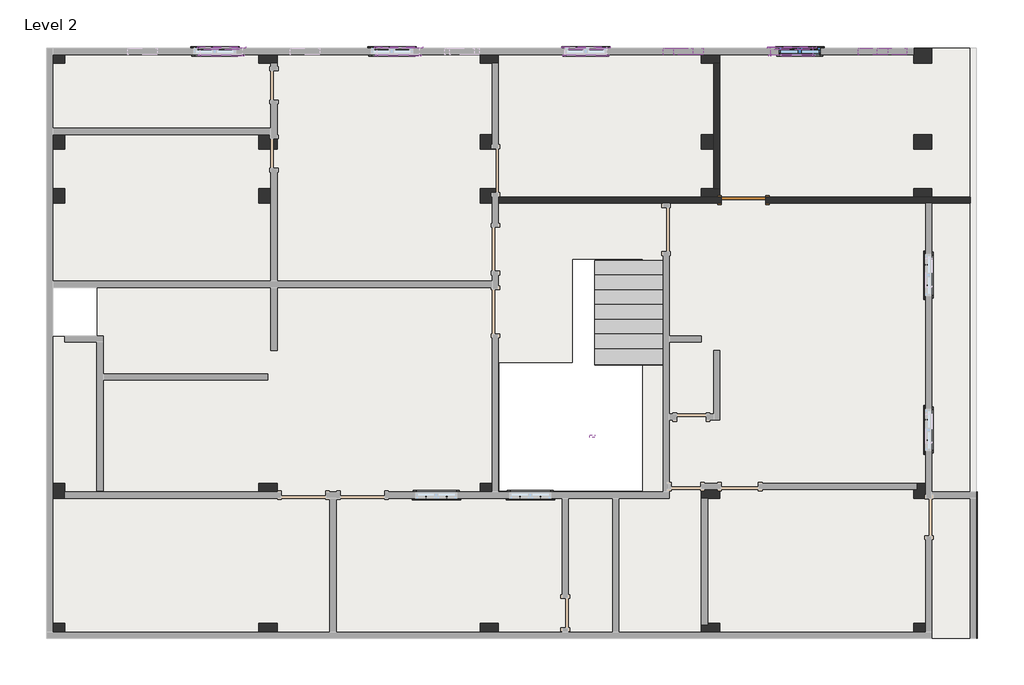
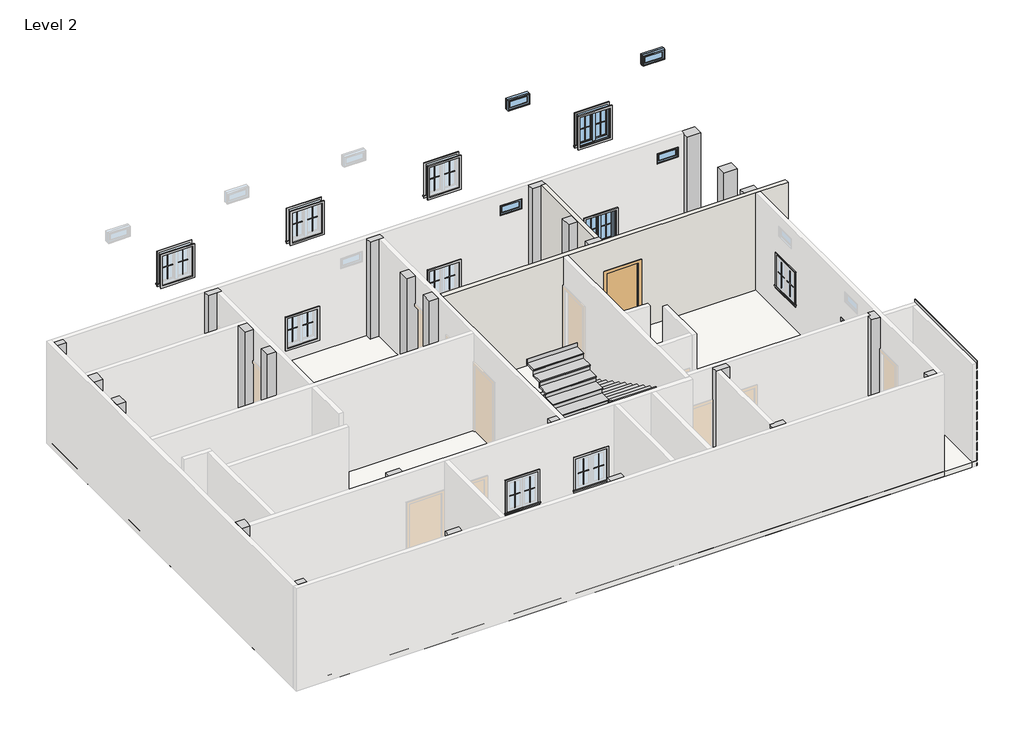
# One storey, part 2 of 2: 48 proxies, 25 columns, 6 windows, 2 walls, 1 air terminal, 1 door, 1 member, 1 slab, 1 stair flight.
"""IFC4 building model written with IfcOpenShell, lengths in millimetres."""

from ifc_helpers import new_model, si_unit, frame, origin, place, context, project, spatial, polyline, outline, extrude, faceted_brep, transform, mapped, element, save
from components import air_terminals_1_air_terminals_1_05a11ed2, muntin_pattern_2x2_muntin_pattern_2x2_b3fe6957, muntin_pattern_2x2_muntin_pattern_2x2_3e0ecaf2, trim_window_exterior_flat_with_sill_41619996, trim_window_interior_flat_picture_frame_51c85655, door_a3eb833a, stair_flight_69588459, window_4c2727af, window_0d9958e7

model = new_model("IFC4")

# Units and contexts
model_context = context("Model", 3, world=origin())
ifc_project = project(units=[si_unit("LENGTHUNIT", "METRE", prefix="MILLI")], contexts=[model_context])

# Site, building, storey
site = spatial("IfcSite", under=ifc_project)
building = spatial("IfcBuilding", under=site)
storey = spatial("IfcBuildingStorey", under=building, Name="Level 2", Elevation=3048.0)

# Air terminal
placement = place(None, origin())
air_terminals_1_air_terminals_1_shape = air_terminals_1_air_terminals_1_05a11ed2(model_context)
element("IfcAirTerminal", 1, ObjectType="Air Terminals 1 : Air Terminals 1", at=placement, inside=storey, context=model_context, shape_type="MappedRepresentation", body=[
    mapped(air_terminals_1_air_terminals_1_shape, transform((0.0, 0.0, 0.0), x_axis=(1.0, 0.0, 0.0), y_axis=(0.0, 1.0, 0.0), z_axis=(0.0, 0.0, 1.0))),
])

# Proxies
muntin_pattern_2x2_muntin_pattern_2x2_shape = muntin_pattern_2x2_muntin_pattern_2x2_b3fe6957(model_context)
element("IfcBuildingElementProxy", 2, Name="Muntin Pattern_2x2 : Muntin Pattern_2x2", ObjectType="Muntin Pattern_2x2 : Muntin Pattern_2x2", at=placement, inside=storey, context=model_context, shape_type="MappedRepresentation", body=[
    mapped(muntin_pattern_2x2_muntin_pattern_2x2_shape, transform((-4178.9300534, -6055.6581508, 4032.25), x_axis=(-1.0, 0.0, 0.0), y_axis=(0.0, -1.0, 0.0), z_axis=(0.0, 0.0, 1.0))),
])
element("IfcBuildingElementProxy", 3, Name="Muntin Pattern_2x2 : Muntin Pattern_2x2", ObjectType="Muntin Pattern_2x2 : Muntin Pattern_2x2", at=placement, inside=storey, context=model_context, shape_type="MappedRepresentation", body=[
    mapped(muntin_pattern_2x2_muntin_pattern_2x2_shape, transform((-2238.8239737, -6055.6581508, 4032.25), x_axis=(-1.0, 0.0, 0.0), y_axis=(0.0, -1.0, 0.0), z_axis=(0.0, 0.0, 1.0))),
])
element("IfcBuildingElementProxy", 4, Name="Muntin Pattern_2x2 : Muntin Pattern_2x2", ObjectType="Muntin Pattern_2x2 : Muntin Pattern_2x2", at=placement, inside=storey, context=model_context, shape_type="MappedRepresentation", body=[
    mapped(muntin_pattern_2x2_muntin_pattern_2x2_shape, transform((5725.4824466, -4869.7956508, 4032.25), x_axis=(0.0, 1.0, 0.0), y_axis=(-1.0, 0.0, 0.0), z_axis=(0.0, 0.0, 1.0))),
])
element("IfcBuildingElementProxy", 5, Name="Muntin Pattern_2x2 : Muntin Pattern_2x2", ObjectType="Muntin Pattern_2x2 : Muntin Pattern_2x2", at=placement, inside=storey, context=model_context, shape_type="MappedRepresentation", body=[
    mapped(muntin_pattern_2x2_muntin_pattern_2x2_shape, transform((5725.4824466, -1669.3956508, 4032.25), x_axis=(0.0, 1.0, 0.0), y_axis=(-1.0, 0.0, 0.0), z_axis=(0.0, 0.0, 1.0))),
])
element("IfcBuildingElementProxy", 6, Name="Muntin Pattern_2x2 : Muntin Pattern_2x2", ObjectType="Muntin Pattern_2x2 : Muntin Pattern_2x2", at=placement, inside=storey, context=model_context, shape_type="MappedRepresentation", body=[
    mapped(muntin_pattern_2x2_muntin_pattern_2x2_shape, transform((2733.0449466, 3221.6918492, 6774.3523039), x_axis=(1.0, 0.0, 0.0), y_axis=(0.0, 1.0, 0.0), z_axis=(0.0, 0.0, 1.0))),
])
element("IfcBuildingElementProxy", 7, Name="Muntin Pattern_2x2 : Muntin Pattern_2x2", ObjectType="Muntin Pattern_2x2 : Muntin Pattern_2x2", at=placement, inside=storey, context=model_context, shape_type="MappedRepresentation", body=[
    mapped(muntin_pattern_2x2_muntin_pattern_2x2_shape, transform((-1521.092894, 3221.6918492, 6774.3523039), x_axis=(1.0, 0.0, 0.0), y_axis=(0.0, 1.0, 0.0), z_axis=(0.0, 0.0, 1.0))),
])
element("IfcBuildingElementProxy", 8, Name="Muntin Pattern_2x2 : Muntin Pattern_2x2", ObjectType="Muntin Pattern_2x2 : Muntin Pattern_2x2", at=placement, inside=storey, context=model_context, shape_type="MappedRepresentation", body=[
    mapped(muntin_pattern_2x2_muntin_pattern_2x2_shape, transform((-1521.092894, 3221.6918492, 3670.3), x_axis=(1.0, 0.0, 0.0), y_axis=(0.0, 1.0, 0.0), z_axis=(0.0, 0.0, 1.0))),
])
element("IfcBuildingElementProxy", 9, Name="Muntin Pattern_2x2 : Muntin Pattern_2x2", ObjectType="Muntin Pattern_2x2 : Muntin Pattern_2x2", at=placement, inside=storey, context=model_context, shape_type="MappedRepresentation", body=[
    mapped(muntin_pattern_2x2_muntin_pattern_2x2_shape, transform((2898.507106, 3221.6918492, 3670.3), x_axis=(1.0, 0.0, 0.0), y_axis=(0.0, 1.0, 0.0), z_axis=(0.0, 0.0, 1.0))),
])
element("IfcBuildingElementProxy", 10, Name="Muntin Pattern_2x2 : Muntin Pattern_2x2", ObjectType="Muntin Pattern_2x2 : Muntin Pattern_2x2", at=placement, inside=storey, context=model_context, shape_type="MappedRepresentation", body=[
    mapped(muntin_pattern_2x2_muntin_pattern_2x2_shape, transform((-5391.7800534, 3221.6918492, 6774.3523039), x_axis=(1.0, 0.0, 0.0), y_axis=(0.0, 1.0, 0.0), z_axis=(0.0, 0.0, 1.0))),
])
element("IfcBuildingElementProxy", 11, Name="Muntin Pattern_2x2 : Muntin Pattern_2x2", ObjectType="Muntin Pattern_2x2 : Muntin Pattern_2x2", at=placement, inside=storey, context=model_context, shape_type="MappedRepresentation", body=[
    mapped(muntin_pattern_2x2_muntin_pattern_2x2_shape, transform((-9049.3800534, 3221.6918492, 6774.3523039), x_axis=(1.0, 0.0, 0.0), y_axis=(0.0, 1.0, 0.0), z_axis=(0.0, 0.0, 1.0))),
])
element("IfcBuildingElementProxy", 12, Name="Muntin Pattern_2x2 : Muntin Pattern_2x2", ObjectType="Muntin Pattern_2x2 : Muntin Pattern_2x2", at=placement, inside=storey, context=model_context, shape_type="MappedRepresentation", body=[
    mapped(muntin_pattern_2x2_muntin_pattern_2x2_shape, transform((-5525.1300534, 3221.6918492, 3670.3), x_axis=(1.0, 0.0, 0.0), y_axis=(0.0, 1.0, 0.0), z_axis=(0.0, 0.0, 1.0))),
])
element("IfcBuildingElementProxy", 13, Name="Muntin Pattern_2x2 : Muntin Pattern_2x2", ObjectType="Muntin Pattern_2x2 : Muntin Pattern_2x2", at=placement, inside=storey, context=model_context, shape_type="MappedRepresentation", body=[
    mapped(muntin_pattern_2x2_muntin_pattern_2x2_shape, transform((-9182.7300534, 3221.6918492, 3670.3), x_axis=(1.0, 0.0, 0.0), y_axis=(0.0, 1.0, 0.0), z_axis=(0.0, 0.0, 1.0))),
])
muntin_pattern_2x2_muntin_pattern_2x2_2_shape = muntin_pattern_2x2_muntin_pattern_2x2_3e0ecaf2(model_context)
element("IfcBuildingElementProxy", 14, Name="Muntin Pattern_2x2 : Muntin Pattern_2x2", ObjectType="Muntin Pattern_2x2 : Muntin Pattern_2x2", at=placement, inside=storey, context=model_context, shape_type="MappedRepresentation", body=[
    mapped(muntin_pattern_2x2_muntin_pattern_2x2_2_shape, transform((-4607.5550534, -6055.6581508, 4032.25), x_axis=(1.0, 0.0, 0.0), y_axis=(0.0, 1.0, 0.0), z_axis=(0.0, 0.0, 1.0))),
])
element("IfcBuildingElementProxy", 15, Name="Muntin Pattern_2x2 : Muntin Pattern_2x2", ObjectType="Muntin Pattern_2x2 : Muntin Pattern_2x2", at=placement, inside=storey, context=model_context, shape_type="MappedRepresentation", body=[
    mapped(muntin_pattern_2x2_muntin_pattern_2x2_2_shape, transform((-2667.4489737, -6055.6581508, 4032.25), x_axis=(1.0, 0.0, 0.0), y_axis=(0.0, 1.0, 0.0), z_axis=(0.0, 0.0, 1.0))),
])
element("IfcBuildingElementProxy", 16, Name="Muntin Pattern_2x2 : Muntin Pattern_2x2", ObjectType="Muntin Pattern_2x2 : Muntin Pattern_2x2", at=placement, inside=storey, context=model_context, shape_type="MappedRepresentation", body=[
    mapped(muntin_pattern_2x2_muntin_pattern_2x2_2_shape, transform((5725.4824466, -4441.1706508, 4032.25), x_axis=(0.0, -1.0, 0.0), y_axis=(1.0, 0.0, 0.0), z_axis=(0.0, 0.0, 1.0))),
])
element("IfcBuildingElementProxy", 17, Name="Muntin Pattern_2x2 : Muntin Pattern_2x2", ObjectType="Muntin Pattern_2x2 : Muntin Pattern_2x2", at=placement, inside=storey, context=model_context, shape_type="MappedRepresentation", body=[
    mapped(muntin_pattern_2x2_muntin_pattern_2x2_2_shape, transform((5725.4824466, -1240.7706508, 4032.25), x_axis=(0.0, -1.0, 0.0), y_axis=(1.0, 0.0, 0.0), z_axis=(0.0, 0.0, 1.0))),
])
element("IfcBuildingElementProxy", 18, Name="Muntin Pattern_2x2 : Muntin Pattern_2x2", ObjectType="Muntin Pattern_2x2 : Muntin Pattern_2x2", at=placement, inside=storey, context=model_context, shape_type="MappedRepresentation", body=[
    mapped(muntin_pattern_2x2_muntin_pattern_2x2_2_shape, transform((3161.6699466, 3221.6918492, 6774.3523039), x_axis=(-1.0, 0.0, 0.0), y_axis=(0.0, -1.0, 0.0), z_axis=(0.0, 0.0, 1.0))),
])
element("IfcBuildingElementProxy", 19, Name="Muntin Pattern_2x2 : Muntin Pattern_2x2", ObjectType="Muntin Pattern_2x2 : Muntin Pattern_2x2", at=placement, inside=storey, context=model_context, shape_type="MappedRepresentation", body=[
    mapped(muntin_pattern_2x2_muntin_pattern_2x2_2_shape, transform((-1092.467894, 3221.6918492, 6774.3523039), x_axis=(-1.0, 0.0, 0.0), y_axis=(0.0, -1.0, 0.0), z_axis=(0.0, 0.0, 1.0))),
])
element("IfcBuildingElementProxy", 20, Name="Muntin Pattern_2x2 : Muntin Pattern_2x2", ObjectType="Muntin Pattern_2x2 : Muntin Pattern_2x2", at=placement, inside=storey, context=model_context, shape_type="MappedRepresentation", body=[
    mapped(muntin_pattern_2x2_muntin_pattern_2x2_2_shape, transform((-1092.467894, 3221.6918492, 3670.3), x_axis=(-1.0, 0.0, 0.0), y_axis=(0.0, -1.0, 0.0), z_axis=(0.0, 0.0, 1.0))),
])
element("IfcBuildingElementProxy", 21, Name="Muntin Pattern_2x2 : Muntin Pattern_2x2", ObjectType="Muntin Pattern_2x2 : Muntin Pattern_2x2", at=placement, inside=storey, context=model_context, shape_type="MappedRepresentation", body=[
    mapped(muntin_pattern_2x2_muntin_pattern_2x2_2_shape, transform((3327.132106, 3221.6918492, 3670.3), x_axis=(-1.0, 0.0, 0.0), y_axis=(0.0, -1.0, 0.0), z_axis=(0.0, 0.0, 1.0))),
])
element("IfcBuildingElementProxy", 22, Name="Muntin Pattern_2x2 : Muntin Pattern_2x2", ObjectType="Muntin Pattern_2x2 : Muntin Pattern_2x2", at=placement, inside=storey, context=model_context, shape_type="MappedRepresentation", body=[
    mapped(muntin_pattern_2x2_muntin_pattern_2x2_2_shape, transform((-4963.1550534, 3221.6918492, 6774.3523039), x_axis=(-1.0, 0.0, 0.0), y_axis=(0.0, -1.0, 0.0), z_axis=(0.0, 0.0, 1.0))),
])
element("IfcBuildingElementProxy", 23, Name="Muntin Pattern_2x2 : Muntin Pattern_2x2", ObjectType="Muntin Pattern_2x2 : Muntin Pattern_2x2", at=placement, inside=storey, context=model_context, shape_type="MappedRepresentation", body=[
    mapped(muntin_pattern_2x2_muntin_pattern_2x2_2_shape, transform((-8620.7550534, 3221.6918492, 6774.3523039), x_axis=(-1.0, 0.0, 0.0), y_axis=(0.0, -1.0, 0.0), z_axis=(0.0, 0.0, 1.0))),
])
element("IfcBuildingElementProxy", 24, Name="Muntin Pattern_2x2 : Muntin Pattern_2x2", ObjectType="Muntin Pattern_2x2 : Muntin Pattern_2x2", at=placement, inside=storey, context=model_context, shape_type="MappedRepresentation", body=[
    mapped(muntin_pattern_2x2_muntin_pattern_2x2_2_shape, transform((-5096.5050534, 3221.6918492, 3670.3), x_axis=(-1.0, 0.0, 0.0), y_axis=(0.0, -1.0, 0.0), z_axis=(0.0, 0.0, 1.0))),
])
element("IfcBuildingElementProxy", 25, Name="Muntin Pattern_2x2 : Muntin Pattern_2x2", ObjectType="Muntin Pattern_2x2 : Muntin Pattern_2x2", at=placement, inside=storey, context=model_context, shape_type="MappedRepresentation", body=[
    mapped(muntin_pattern_2x2_muntin_pattern_2x2_2_shape, transform((-8754.1050534, 3221.6918492, 3670.3), x_axis=(-1.0, 0.0, 0.0), y_axis=(0.0, -1.0, 0.0), z_axis=(0.0, 0.0, 1.0))),
])
trim_window_exterior_flat_with_sill_shape = trim_window_exterior_flat_with_sill_41619996(model_context)
element("IfcBuildingElementProxy", 26, Name="Trim-Window-Exterior-Flat : with Sill", ObjectType="Trim-Window-Exterior-Flat : with Sill", at=placement, inside=storey, context=model_context, shape_type="MappedRepresentation", body=[
    mapped(trim_window_exterior_flat_with_sill_shape, transform((-4393.2425534, -6065.1831508, 4876.8), x_axis=(1.0, 0.0, 0.0), y_axis=(0.0, 0.0, 1.0), z_axis=(0.0, -1.0, 0.0))),
])
element("IfcBuildingElementProxy", 27, Name="Trim-Window-Exterior-Flat : with Sill", ObjectType="Trim-Window-Exterior-Flat : with Sill", at=placement, inside=storey, context=model_context, shape_type="MappedRepresentation", body=[
    mapped(trim_window_exterior_flat_with_sill_shape, transform((-2453.1364737, -6065.1831508, 4876.8), x_axis=(1.0, 0.0, 0.0), y_axis=(0.0, 0.0, 1.0), z_axis=(0.0, -1.0, 0.0))),
])
element("IfcBuildingElementProxy", 28, Name="Trim-Window-Exterior-Flat : with Sill", ObjectType="Trim-Window-Exterior-Flat : with Sill", at=placement, inside=storey, context=model_context, shape_type="MappedRepresentation", body=[
    mapped(trim_window_exterior_flat_with_sill_shape, transform((5715.9574466, -4655.4831508, 4876.8), x_axis=(0.0, -1.0, 0.0), y_axis=(0.0, 0.0, 1.0), z_axis=(-1.0, 0.0, 0.0))),
])
element("IfcBuildingElementProxy", 29, Name="Trim-Window-Exterior-Flat : with Sill", ObjectType="Trim-Window-Exterior-Flat : with Sill", at=placement, inside=storey, context=model_context, shape_type="MappedRepresentation", body=[
    mapped(trim_window_exterior_flat_with_sill_shape, transform((5715.9574466, -1455.0831508, 4876.8), x_axis=(0.0, -1.0, 0.0), y_axis=(0.0, 0.0, 1.0), z_axis=(-1.0, 0.0, 0.0))),
])
element("IfcBuildingElementProxy", 30, Name="Trim-Window-Exterior-Flat : with Sill", ObjectType="Trim-Window-Exterior-Flat : with Sill", at=placement, inside=storey, context=model_context, shape_type="MappedRepresentation", body=[
    mapped(trim_window_exterior_flat_with_sill_shape, transform((2947.3574466, 3231.2168492, 7618.9023039), x_axis=(-1.0, 0.0, 0.0), y_axis=(0.0, 0.0, 1.0), z_axis=(0.0, 1.0, 0.0))),
])
element("IfcBuildingElementProxy", 31, Name="Trim-Window-Exterior-Flat : with Sill", ObjectType="Trim-Window-Exterior-Flat : with Sill", at=placement, inside=storey, context=model_context, shape_type="MappedRepresentation", body=[
    mapped(trim_window_exterior_flat_with_sill_shape, transform((-1306.780394, 3231.2168492, 7618.9023039), x_axis=(-1.0, 0.0, 0.0), y_axis=(0.0, 0.0, 1.0), z_axis=(0.0, 1.0, 0.0))),
])
element("IfcBuildingElementProxy", 32, Name="Trim-Window-Exterior-Flat : with Sill", ObjectType="Trim-Window-Exterior-Flat : with Sill", at=placement, inside=storey, context=model_context, shape_type="MappedRepresentation", body=[
    mapped(trim_window_exterior_flat_with_sill_shape, transform((-1306.780394, 3231.2168492, 4514.85), x_axis=(-1.0, 0.0, 0.0), y_axis=(0.0, 0.0, 1.0), z_axis=(0.0, 1.0, 0.0))),
])
element("IfcBuildingElementProxy", 33, Name="Trim-Window-Exterior-Flat : with Sill", ObjectType="Trim-Window-Exterior-Flat : with Sill", at=placement, inside=storey, context=model_context, shape_type="MappedRepresentation", body=[
    mapped(trim_window_exterior_flat_with_sill_shape, transform((3112.819606, 3231.2168492, 4514.85), x_axis=(-1.0, 0.0, 0.0), y_axis=(0.0, 0.0, 1.0), z_axis=(0.0, 1.0, 0.0))),
])
element("IfcBuildingElementProxy", 34, Name="Trim-Window-Exterior-Flat : with Sill", ObjectType="Trim-Window-Exterior-Flat : with Sill", at=placement, inside=storey, context=model_context, shape_type="MappedRepresentation", body=[
    mapped(trim_window_exterior_flat_with_sill_shape, transform((-5177.4675534, 3231.2168492, 7618.9023039), x_axis=(-1.0, 0.0, 0.0), y_axis=(0.0, 0.0, 1.0), z_axis=(0.0, 1.0, 0.0))),
])
element("IfcBuildingElementProxy", 35, Name="Trim-Window-Exterior-Flat : with Sill", ObjectType="Trim-Window-Exterior-Flat : with Sill", at=placement, inside=storey, context=model_context, shape_type="MappedRepresentation", body=[
    mapped(trim_window_exterior_flat_with_sill_shape, transform((-8835.0675534, 3231.2168492, 7618.9023039), x_axis=(-1.0, 0.0, 0.0), y_axis=(0.0, 0.0, 1.0), z_axis=(0.0, 1.0, 0.0))),
])
element("IfcBuildingElementProxy", 36, Name="Trim-Window-Exterior-Flat : with Sill", ObjectType="Trim-Window-Exterior-Flat : with Sill", at=placement, inside=storey, context=model_context, shape_type="MappedRepresentation", body=[
    mapped(trim_window_exterior_flat_with_sill_shape, transform((-5310.8175534, 3231.2168492, 4514.85), x_axis=(-1.0, 0.0, 0.0), y_axis=(0.0, 0.0, 1.0), z_axis=(0.0, 1.0, 0.0))),
])
element("IfcBuildingElementProxy", 37, Name="Trim-Window-Exterior-Flat : with Sill", ObjectType="Trim-Window-Exterior-Flat : with Sill", at=placement, inside=storey, context=model_context, shape_type="MappedRepresentation", body=[
    mapped(trim_window_exterior_flat_with_sill_shape, transform((-8968.4175534, 3231.2168492, 4514.85), x_axis=(-1.0, 0.0, 0.0), y_axis=(0.0, 0.0, 1.0), z_axis=(0.0, 1.0, 0.0))),
])
trim_window_interior_flat_picture_frame_shape = trim_window_interior_flat_picture_frame_51c85655(model_context)
element("IfcBuildingElementProxy", 38, Name="Trim-Window-Interior-Flat : Picture Frame", ObjectType="Trim-Window-Interior-Flat : Picture Frame", at=placement, inside=storey, context=model_context, shape_type="MappedRepresentation", body=[
    mapped(trim_window_interior_flat_picture_frame_shape, transform((-4393.2425534, -5938.1831508, 4876.8), x_axis=(-1.0, 0.0, 0.0), y_axis=(0.0, 0.0, 1.0), z_axis=(0.0, 1.0, 0.0))),
])
element("IfcBuildingElementProxy", 39, Name="Trim-Window-Interior-Flat : Picture Frame", ObjectType="Trim-Window-Interior-Flat : Picture Frame", at=placement, inside=storey, context=model_context, shape_type="MappedRepresentation", body=[
    mapped(trim_window_interior_flat_picture_frame_shape, transform((-2453.1364737, -5938.1831508, 4876.8), x_axis=(-1.0, 0.0, 0.0), y_axis=(0.0, 0.0, 1.0), z_axis=(0.0, 1.0, 0.0))),
])
element("IfcBuildingElementProxy", 40, Name="Trim-Window-Interior-Flat : Picture Frame", ObjectType="Trim-Window-Interior-Flat : Picture Frame", at=placement, inside=storey, context=model_context, shape_type="MappedRepresentation", body=[
    mapped(trim_window_interior_flat_picture_frame_shape, transform((5842.9574466, -4655.4831508, 4876.8), x_axis=(0.0, 1.0, 0.0), y_axis=(0.0, 0.0, 1.0), z_axis=(1.0, 0.0, 0.0))),
])
element("IfcBuildingElementProxy", 41, Name="Trim-Window-Interior-Flat : Picture Frame", ObjectType="Trim-Window-Interior-Flat : Picture Frame", at=placement, inside=storey, context=model_context, shape_type="MappedRepresentation", body=[
    mapped(trim_window_interior_flat_picture_frame_shape, transform((5842.9574466, -1455.0831508, 4876.8), x_axis=(0.0, 1.0, 0.0), y_axis=(0.0, 0.0, 1.0), z_axis=(1.0, 0.0, 0.0))),
])
element("IfcBuildingElementProxy", 42, Name="Trim-Window-Interior-Flat : Picture Frame", ObjectType="Trim-Window-Interior-Flat : Picture Frame", at=placement, inside=storey, context=model_context, shape_type="MappedRepresentation", body=[
    mapped(trim_window_interior_flat_picture_frame_shape, transform((2947.3574466, 3104.2168492, 7618.9023039), x_axis=(1.0, 0.0, 0.0), y_axis=(0.0, 0.0, 1.0), z_axis=(0.0, -1.0, 0.0))),
])
element("IfcBuildingElementProxy", 43, Name="Trim-Window-Interior-Flat : Picture Frame", ObjectType="Trim-Window-Interior-Flat : Picture Frame", at=placement, inside=storey, context=model_context, shape_type="MappedRepresentation", body=[
    mapped(trim_window_interior_flat_picture_frame_shape, transform((-1306.780394, 3104.2168492, 7618.9023039), x_axis=(1.0, 0.0, 0.0), y_axis=(0.0, 0.0, 1.0), z_axis=(0.0, -1.0, 0.0))),
])
element("IfcBuildingElementProxy", 44, Name="Trim-Window-Interior-Flat : Picture Frame", ObjectType="Trim-Window-Interior-Flat : Picture Frame", at=placement, inside=storey, context=model_context, shape_type="MappedRepresentation", body=[
    mapped(trim_window_interior_flat_picture_frame_shape, transform((-1306.780394, 3104.2168492, 4514.85), x_axis=(1.0, 0.0, 0.0), y_axis=(0.0, 0.0, 1.0), z_axis=(0.0, -1.0, 0.0))),
])
element("IfcBuildingElementProxy", 45, Name="Trim-Window-Interior-Flat : Picture Frame", ObjectType="Trim-Window-Interior-Flat : Picture Frame", at=placement, inside=storey, context=model_context, shape_type="MappedRepresentation", body=[
    mapped(trim_window_interior_flat_picture_frame_shape, transform((3112.819606, 3104.2168492, 4514.85), x_axis=(1.0, 0.0, 0.0), y_axis=(0.0, 0.0, 1.0), z_axis=(0.0, -1.0, 0.0))),
])
element("IfcBuildingElementProxy", 46, Name="Trim-Window-Interior-Flat : Picture Frame", ObjectType="Trim-Window-Interior-Flat : Picture Frame", at=placement, inside=storey, context=model_context, shape_type="MappedRepresentation", body=[
    mapped(trim_window_interior_flat_picture_frame_shape, transform((-5177.4675534, 3104.2168492, 7618.9023039), x_axis=(1.0, 0.0, 0.0), y_axis=(0.0, 0.0, 1.0), z_axis=(0.0, -1.0, 0.0))),
])
element("IfcBuildingElementProxy", 47, Name="Trim-Window-Interior-Flat : Picture Frame", ObjectType="Trim-Window-Interior-Flat : Picture Frame", at=placement, inside=storey, context=model_context, shape_type="MappedRepresentation", body=[
    mapped(trim_window_interior_flat_picture_frame_shape, transform((-8835.0675534, 3104.2168492, 7618.9023039), x_axis=(1.0, 0.0, 0.0), y_axis=(0.0, 0.0, 1.0), z_axis=(0.0, -1.0, 0.0))),
])
element("IfcBuildingElementProxy", 48, Name="Trim-Window-Interior-Flat : Picture Frame", ObjectType="Trim-Window-Interior-Flat : Picture Frame", at=placement, inside=storey, context=model_context, shape_type="MappedRepresentation", body=[
    mapped(trim_window_interior_flat_picture_frame_shape, transform((-5310.8175534, 3104.2168492, 4514.85), x_axis=(1.0, 0.0, 0.0), y_axis=(0.0, 0.0, 1.0), z_axis=(0.0, -1.0, 0.0))),
])
element("IfcBuildingElementProxy", 49, Name="Trim-Window-Interior-Flat : Picture Frame", ObjectType="Trim-Window-Interior-Flat : Picture Frame", at=placement, inside=storey, context=model_context, shape_type="MappedRepresentation", body=[
    mapped(trim_window_interior_flat_picture_frame_shape, transform((-8968.4175534, 3104.2168492, 4514.85), x_axis=(1.0, 0.0, 0.0), y_axis=(0.0, 0.0, 1.0), z_axis=(0.0, -1.0, 0.0))),
])

# Columns
element("IfcColumn", 50, ObjectType="column family : column family", at=placement, inside=storey, context=model_context, shape_type="SweptSolid", body=[
    extrude(outline(polyline([(-12064.0425534, 2926.4168492), (-12318.0425534, 2926.4168492), (-12318.0425534, 3104.2168492), (-12064.0425534, 3104.2168492), (-12064.0425534, 2926.4168492)])), frame((0.0, 0.0, 3053.0), z_axis=(0.0, 0.0, 1.0), x_axis=(1.0, 0.0, 0.0)), (0.0, 0.0, 1.0), 3038.0),
])
element("IfcColumn", 51, ObjectType="column family : column family", at=placement, inside=storey, context=model_context, shape_type="SweptSolid", body=[
    extrude(outline(polyline([(-7682.5425534, 2926.4168492), (-8063.5425534, 2926.4168492), (-8063.5425534, 3104.2168492), (-7682.5425534, 3104.2168492), (-7682.5425534, 2926.4168492)])), frame((0.0, 0.0, 3053.0), z_axis=(0.0, 0.0, 1.0), x_axis=(1.0, 0.0, 0.0)), (0.0, 0.0, 1.0), 3038.0),
])
element("IfcColumn", 52, ObjectType="column family : column family", at=placement, inside=storey, context=model_context, shape_type="SweptSolid", body=[
    extrude(outline(polyline([(-3110.5425534, 2926.4168492), (-3491.5425534, 2926.4168492), (-3491.5425534, 3104.2168492), (-3110.5425534, 3104.2168492), (-3110.5425534, 2926.4168492)])), frame((0.0, 0.0, 3053.0), z_axis=(0.0, 0.0, 1.0), x_axis=(1.0, 0.0, 0.0)), (0.0, 0.0, 1.0), 3038.0),
])
element("IfcColumn", 53, ObjectType="column family : column family", at=placement, inside=storey, context=model_context, shape_type="SweptSolid", body=[
    extrude(outline(polyline([(1461.4574466, 2926.4168492), (1080.4574466, 2926.4168492), (1080.4574466, 3104.2168492), (1461.4574466, 3104.2168492), (1461.4574466, 2926.4168492)])), frame((0.0, 0.0, 3053.0), z_axis=(0.0, 0.0, 1.0), x_axis=(1.0, 0.0, 0.0)), (0.0, 0.0, 1.0), 3038.0),
])
element("IfcColumn", 54, ObjectType="column family : column family", at=placement, inside=storey, context=model_context, shape_type="SweptSolid", body=[
    extrude(outline(polyline([(5842.9574466, 3231.2168492), (5842.9574466, 2926.4168492), (5461.9574466, 2926.4168492), (5461.9574466, 3231.2168492), (5842.9574466, 3231.2168492)])), frame((0.0, 0.0, 3053.0), z_axis=(0.0, 0.0, 1.0), x_axis=(1.0, 0.0, 0.0)), (0.0, 0.0, 1.0), 3038.0),
])
element("IfcColumn", 55, ObjectType="column family : column family", at=placement, inside=storey, context=model_context, shape_type="SweptSolid", body=[
    extrude(outline(polyline([(-12064.0425534, 335.6168492), (-12064.0425534, 30.8168492), (-12318.0425534, 30.8168492), (-12318.0425534, 335.6168492), (-12064.0425534, 335.6168492)])), frame((0.0, 0.0, 3053.0), z_axis=(0.0, 0.0, 1.0), x_axis=(1.0, 0.0, 0.0)), (0.0, 0.0, 1.0), 3038.0),
])
element("IfcColumn", 56, ObjectType="column family : column family", at=placement, inside=storey, context=model_context, shape_type="SweptSolid", body=[
    extrude(outline(polyline([(-12064.0425534, 1449.6754758), (-12064.0425534, 1144.8754758), (-12318.0425534, 1144.8754758), (-12318.0425534, 1449.6754758), (-12064.0425534, 1449.6754758)])), frame((0.0, 0.0, 3053.0), z_axis=(0.0, 0.0, 1.0), x_axis=(1.0, 0.0, 0.0)), (0.0, 0.0, 1.0), 3038.0),
])
element("IfcColumn", 57, ObjectType="column family : column family", at=placement, inside=storey, context=model_context, shape_type="SweptSolid", body=[
    extrude(outline(polyline([(-12064.0425534, -5760.3831508), (-12064.0425534, -6065.1831508), (-12318.0425534, -6065.1831508), (-12318.0425534, -5760.3831508), (-12064.0425534, -5760.3831508)])), frame((0.0, 0.0, 3053.0), z_axis=(0.0, 0.0, 1.0), x_axis=(1.0, 0.0, 0.0)), (0.0, 0.0, 1.0), 3038.0),
])
element("IfcColumn", 58, ObjectType="column family : column family", at=placement, inside=storey, context=model_context, shape_type="SweptSolid", body=[
    extrude(outline(polyline([(-12064.0425534, -8655.9831508), (-12064.0425534, -8833.7831508), (-12318.0425534, -8833.7831508), (-12318.0425534, -8655.9831508), (-12064.0425534, -8655.9831508)])), frame((0.0, 0.0, 3053.0), z_axis=(0.0, 0.0, 1.0), x_axis=(1.0, 0.0, 0.0)), (0.0, 0.0, 1.0), 3038.0),
])
element("IfcColumn", 59, ObjectType="column family : column family", at=placement, inside=storey, context=model_context, shape_type="SweptSolid", body=[
    extrude(outline(polyline([(5461.9574466, 335.6168492), (5842.9574466, 335.6168492), (5842.9574466, 157.8168492), (5461.9574466, 157.8168492), (5461.9574466, 335.6168492)])), frame((0.0, 0.0, 3053.0), z_axis=(0.0, 0.0, 1.0), x_axis=(1.0, 0.0, 0.0)), (0.0, 0.0, 1.0), 3038.0),
])
element("IfcColumn", 60, ObjectType="column family : column family", at=placement, inside=storey, context=model_context, shape_type="SweptSolid", body=[
    extrude(outline(polyline([(5842.9574466, 1449.6754758), (5842.9574466, 1144.8754758), (5461.9574466, 1144.8754758), (5461.9574466, 1449.6754758), (5842.9574466, 1449.6754758)])), frame((0.0, 0.0, 3053.0), z_axis=(0.0, 0.0, 1.0), x_axis=(1.0, 0.0, 0.0)), (0.0, 0.0, 1.0), 3038.0),
])
element("IfcColumn", 61, ObjectType="column family : column family", at=placement, inside=storey, context=model_context, shape_type="SweptSolid", body=[
    extrude(outline(polyline([(5715.9574466, -6065.1831508), (5461.9574466, -6065.1831508), (5461.9574466, -5887.3831508), (5533.439606, -5887.3831508), (5533.439606, -5760.3831508), (5715.9574466, -5760.3831508), (5715.9574466, -6065.1831508)])), frame((0.0, 0.0, 3053.0), z_axis=(0.0, 0.0, 1.0), x_axis=(1.0, 0.0, 0.0)), (0.0, 0.0, 1.0), 3038.0),
])
element("IfcColumn", 62, ObjectType="column family : column family", at=placement, inside=storey, context=model_context, shape_type="SweptSolid", body=[
    extrude(outline(polyline([(5461.9574466, -8833.7831508), (5461.9574466, -8655.9831508), (5715.9574466, -8655.9831508), (5715.9574466, -8833.7831508), (5461.9574466, -8833.7831508)])), frame((0.0, 0.0, 3053.0), z_axis=(0.0, 0.0, 1.0), x_axis=(1.0, 0.0, 0.0)), (0.0, 0.0, 1.0), 3038.0),
])
element("IfcColumn", 63, ObjectType="column family : column family", at=placement, inside=storey, context=model_context, shape_type="SweptSolid", body=[
    extrude(outline(polyline([(-8063.5425534, -8655.9831508), (-7682.5425534, -8655.9831508), (-7682.5425534, -8833.7831508), (-8063.5425534, -8833.7831508), (-8063.5425534, -8655.9831508)])), frame((0.0, 0.0, 3053.0), z_axis=(0.0, 0.0, 1.0), x_axis=(1.0, 0.0, 0.0)), (0.0, 0.0, 1.0), 3038.0),
])
element("IfcColumn", 64, ObjectType="column family : column family", at=placement, inside=storey, context=model_context, shape_type="SweptSolid", body=[
    extrude(outline(polyline([(-3491.5425534, -8655.9831508), (-3110.5425534, -8655.9831508), (-3110.5425534, -8833.7831508), (-3491.5425534, -8833.7831508), (-3491.5425534, -8655.9831508)])), frame((0.0, 0.0, 3053.0), z_axis=(0.0, 0.0, 1.0), x_axis=(1.0, 0.0, 0.0)), (0.0, 0.0, 1.0), 3038.0),
])
element("IfcColumn", 65, ObjectType="column family : column family", at=placement, inside=storey, context=model_context, shape_type="SweptSolid", body=[
    extrude(outline(polyline([(1461.4574466, -8655.9831508), (1461.4574466, -8833.7831508), (1080.4574466, -8833.7831508), (1080.4574466, -8681.3831508), (1207.4574466, -8681.3831508), (1207.4574466, -8655.9831508), (1461.4574466, -8655.9831508)])), frame((0.0, 0.0, 3053.0), z_axis=(0.0, 0.0, 1.0), x_axis=(1.0, 0.0, 0.0)), (0.0, 0.0, 1.0), 3038.0),
])
element("IfcColumn", 66, ObjectType="column family : column family", at=placement, inside=storey, context=model_context, shape_type="SweptSolid", body=[
    extrude(outline(polyline([(-8063.5425534, 30.8168492), (-8063.5425534, 335.6168492), (-7809.5425534, 335.6168492), (-7809.5425534, 30.8168492), (-8063.5425534, 30.8168492)])), frame((0.0, 0.0, 3053.0), z_axis=(0.0, 0.0, 1.0), x_axis=(1.0, 0.0, 0.0)), (0.0, 0.0, 1.0), 3038.0),
])
element("IfcColumn", 67, ObjectType="column family : column family", at=placement, inside=storey, context=model_context, shape_type="Brep", body=[
    faceted_brep([(-3491.5425534, 30.8168492, 3053.0), (-3491.5425534, 335.6168492, 3053.0), (-3110.5425534, 335.6168492, 3053.0), (-3110.5425534, 246.7168492, 3053.0), (-3237.5425534, 246.7168492, 3053.0), (-3237.5425534, 30.8168492, 3053.0), (-3110.5425534, 335.6168492, 5181.6), (-3110.5425534, 246.7168492, 5181.6), (-3491.5425534, 30.8168492, 6091.0), (-3237.5425534, 30.8168492, 6091.0), (-3491.5425534, 335.6168492, 6091.0), (-3237.5425534, 335.6168492, 6091.0), (-3237.5425534, 335.6168492, 5181.6), (-3237.5425534, 246.7168492, 5181.6)], [[[0, 1, 2, 3, 4, 5]], [[3, 2, 6, 7]], [[8, 0, 5, 9]], [[1, 0, 8, 10]], [[2, 1, 10, 11, 12, 6]], [[10, 8, 9, 11]], [[4, 13, 12, 11, 9, 5]], [[7, 13, 4, 3]], [[13, 7, 6, 12]]]),
])
element("IfcColumn", 68, ObjectType="column family : column family", at=placement, inside=storey, context=model_context, shape_type="SweptSolid", body=[
    extrude(outline(polyline([(1080.4574466, 335.6168492), (1461.4574466, 335.6168492), (1461.4574466, 157.8168492), (1080.4574466, 157.8168492), (1080.4574466, 335.6168492)])), frame((0.0, 0.0, 3053.0), z_axis=(0.0, 0.0, 1.0), x_axis=(1.0, 0.0, 0.0)), (0.0, 0.0, 1.0), 3038.0),
])
element("IfcColumn", 69, ObjectType="column family : column family", at=placement, inside=storey, context=model_context, shape_type="SweptSolid", body=[
    extrude(outline(polyline([(1080.4574466, 1144.8754758), (1080.4574466, 1449.6754758), (1334.4574466, 1449.6754758), (1334.4574466, 1144.8754758), (1080.4574466, 1144.8754758)])), frame((0.0, 0.0, 3053.0), z_axis=(0.0, 0.0, 1.0), x_axis=(1.0, 0.0, 0.0)), (0.0, 0.0, 1.0), 3038.0),
])
element("IfcColumn", 70, ObjectType="column family : column family", at=placement, inside=storey, context=model_context, shape_type="Brep", body=[
    faceted_brep([(-3110.5425534, 1144.8754758, 3053.0), (-3491.5425534, 1144.8754758, 3053.0), (-3491.5425534, 1449.6754758, 3053.0), (-3237.5425534, 1449.6754758, 3053.0), (-3237.5425534, 1161.1168492, 3053.0), (-3110.5425534, 1161.1168492, 3053.0), (-3110.5425534, 1161.1168492, 5181.6), (-3110.5425534, 1144.8754758, 5181.6), (-3237.5425534, 1144.8754758, 5181.6), (-3237.5425534, 1144.8754758, 6091.0), (-3491.5425534, 1144.8754758, 6091.0), (-3491.5425534, 1449.6754758, 6091.0), (-3237.5425534, 1449.6754758, 6091.0), (-3237.5425534, 1161.1168492, 5181.6)], [[[0, 1, 2, 3, 4, 5]], [[0, 5, 6, 7]], [[1, 0, 7, 8, 9, 10]], [[2, 1, 10, 11]], [[2, 11, 12, 3]], [[11, 10, 9, 12]], [[8, 13, 4, 3, 12, 9]], [[6, 13, 8, 7]], [[13, 6, 5, 4]]]),
])
element("IfcColumn", 71, ObjectType="column family : column family", at=placement, inside=storey, context=model_context, shape_type="Brep", body=[
    faceted_brep([(-7682.5425534, 1144.8754758, 3053.0), (-8063.5425534, 1144.8754758, 3053.0), (-8063.5425534, 1449.6754758, 3053.0), (-7809.5425534, 1449.6754758, 3053.0), (-7809.5425534, 1364.3168492, 3053.0), (-7682.5425534, 1364.3168492, 3053.0), (-7682.5425534, 1364.3168492, 5080.0), (-7682.5425534, 1144.8754758, 5080.0), (-7809.5425534, 1144.8754758, 5080.0), (-7809.5425534, 1144.8754758, 6091.0), (-8063.5425534, 1144.8754758, 6091.0), (-8063.5425534, 1449.6754758, 6091.0), (-7809.5425534, 1449.6754758, 6091.0), (-7809.5425534, 1364.3168492, 5080.0)], [[[0, 1, 2, 3, 4, 5]], [[0, 5, 6, 7]], [[1, 0, 7, 8, 9, 10]], [[2, 1, 10, 11]], [[2, 11, 12, 3]], [[11, 10, 9, 12]], [[8, 13, 4, 3, 12, 9]], [[13, 6, 5, 4]], [[6, 13, 8, 7]]]),
])
element("IfcColumn", 72, ObjectType="column family : column family", at=placement, inside=storey, context=model_context, shape_type="SweptSolid", body=[
    extrude(outline(polyline([(-8063.5425534, -5760.3831508), (-7682.5425534, -5760.3831508), (-7682.5425534, -5938.1831508), (-8063.5425534, -5938.1831508), (-8063.5425534, -5760.3831508)])), frame((0.0, 0.0, 3053.0), z_axis=(0.0, 0.0, 1.0), x_axis=(1.0, 0.0, 0.0)), (0.0, 0.0, 1.0), 3038.0),
])
element("IfcColumn", 73, ObjectType="column family : column family", at=placement, inside=storey, context=model_context, shape_type="SweptSolid", body=[
    extrude(outline(polyline([(-3491.5425534, -5760.3831508), (-3237.5425534, -5760.3831508), (-3237.5425534, -5938.1831508), (-3491.5425534, -5938.1831508), (-3491.5425534, -5760.3831508)])), frame((0.0, 0.0, 3053.0), z_axis=(0.0, 0.0, 1.0), x_axis=(1.0, 0.0, 0.0)), (0.0, 0.0, 1.0), 3038.0),
])
element("IfcColumn", 74, ObjectType="column family : column family", at=placement, inside=storey, context=model_context, shape_type="SweptSolid", body=[
    extrude(outline(polyline([(1461.4574466, -6065.1831508), (1080.4574466, -6065.1831508), (1080.4574466, -5887.3831508), (1461.4574466, -5887.3831508), (1461.4574466, -6065.1831508)])), frame((0.0, 0.0, 3053.0), z_axis=(0.0, 0.0, 1.0), x_axis=(1.0, 0.0, 0.0)), (0.0, 0.0, 1.0), 3038.0),
])

# Door
door_shape = door_a3eb833a(model_context)
element("IfcDoor", 75, ObjectType="Single-Flush : 36\" x 84\"", at=placement, inside=storey, context=model_context, shape_type="MappedRepresentation", body=[
    mapped(door_shape, transform((1952.039606, 94.3168492, 3048.0), x_axis=(-1.0, 0.0, 0.0), y_axis=(0.0, -1.0, 0.0), z_axis=(0.0, 0.0, 1.0))),
])

# Member
element("IfcMember", 76, ObjectType="Stringer - 2\" Width", at=placement, inside=storey, context=model_context, shape_type="SweptSolid", body=[
    extrude(outline(polyline([(-1121.360394, -4757.0831508), (-1121.360394, -4807.8831508), (-1222.960394, -4807.8831508), (-1222.960394, -4757.0831508), (-1121.360394, -4757.0831508)])), frame((0.0, 0.0, 4904.8736842), z_axis=(0.0, 0.0, 1.0), x_axis=(1.0, 0.0, 0.0)), (0.0, 0.0, 1.0), 304.8),
])

# Slab
element("IfcSlab", 77, ObjectType="Generic - 12\"", at=placement, inside=storey, context=model_context, shape_type="SweptSolid", body=[
    extrude(outline(polyline([(6757.3574466, 3231.2168492), (6757.3574466, -8960.7831508), (-12445.0425534, -8960.7831508), (-12445.0425534, 3231.2168492), (6757.3574466, 3231.2168492)]), holes=[polyline([(-3096.210394, -5912.7831508), (-144.730394, -5912.7831508), (-144.730394, -1135.0431508), (-1578.560394, -1135.0431508), (-1578.560394, -3273.1068434), (-3096.210394, -3273.1068434), (-3096.210394, -5912.7831508)]), polyline([(-11403.6425534, -1709.0831508), (-12318.0425534, -1709.0831508), (-12318.0425534, -2712.3831508), (-11403.6425534, -2712.3831508), (-11403.6425534, -1709.0831508)])]), frame((0.0, 0.0, 3048.0), z_axis=(0.0, 0.0, 1.0), x_axis=(1.0, 0.0, 0.0)), (0.0, 0.0, 1.0), 152.4),
])

# Stair flight
stair_flight_shape = stair_flight_69588459(model_context)
element("IfcStairFlight", 78, ObjectType="2\" Tread 1\" Nosing 1/4\" Riser", at=placement, inside=storey, context=model_context, shape_type="MappedRepresentation", body=[
    mapped(stair_flight_shape, transform((0.0, 0.0, 0.0), x_axis=(1.0, 0.0, 0.0), y_axis=(0.0, 1.0, 0.0), z_axis=(0.0, 0.0, 1.0))),
])

# Walls
element("IfcWall", 79, ObjectType="Generic - 5\"", at=placement, inside=storey, context=model_context, shape_type="Brep", body=[
    faceted_brep([(-3110.5425534, 30.8168492, 3048.0), (288.339606, 30.8168492, 3048.0), (415.339606, 30.8168492, 3048.0), (1494.839606, 30.8168492, 3048.0), (1494.839606, 30.8168492, 5181.6), (2409.239606, 30.8168492, 5181.6), (2409.239606, 30.8168492, 3048.0), (5715.9574466, 30.8168492, 3048.0), (5842.9574466, 30.8168492, 3048.0), (6630.3574466, 30.8168492, 3048.0), (6630.3574466, 30.8168492, 6096.0), (5842.9574466, 30.8168492, 6096.0), (5715.9574466, 30.8168492, 6096.0), (415.339606, 30.8168492, 6096.0), (288.339606, 30.8168492, 6096.0), (-3110.5425534, 30.8168492, 6096.0), (1494.839606, 157.8168492, 5181.6), (1494.839606, 157.8168492, 3048.0), (-3110.5425534, 157.8168492, 3048.0), (-3110.5425534, 157.8168492, 6096.0), (6630.3574466, 157.8168492, 6096.0), (6630.3574466, 157.8168492, 3048.0), (2409.239606, 157.8168492, 3048.0), (2409.239606, 157.8168492, 5181.6)], [[[0, 1, 2, 3, 4, 5, 6, 7, 8, 9, 10, 11, 12, 13, 14, 15]], [[16, 17, 18, 19, 20, 21, 22, 23]], [[22, 21, 9, 8, 7, 6]], [[18, 17, 3, 2, 1, 0]], [[15, 14, 13, 12, 11, 10, 20, 19]], [[10, 9, 21, 20]], [[0, 15, 19, 18]], [[4, 3, 17, 16]], [[5, 4, 16, 23]], [[6, 5, 23, 22]]]),
])
element("IfcWall", 80, ObjectType="Generic - 5\"", at=placement, inside=storey, context=model_context, shape_type="Brep", body=[
    faceted_brep([(1334.4574466, 2926.4168492, 3048.0), (1334.4574466, 335.6168492, 3048.0), (1334.4574466, 335.6168492, 6096.0), (1334.4574466, 2926.4168492, 6096.0), (1461.4574466, 2926.4168492, 3048.0), (1461.4574466, 2926.4168492, 3053.0), (1461.4574466, 2926.4168492, 6091.0), (1461.4574466, 2926.4168492, 6096.0), (1461.4574466, 335.6168492, 6096.0), (1461.4574466, 335.6168492, 6091.0), (1461.4574466, 335.6168492, 3053.0), (1461.4574466, 335.6168492, 3048.0)], [[[0, 1, 2, 3]], [[4, 5, 6, 7, 8, 9, 10, 11]], [[1, 0, 4, 11]], [[2, 1, 11, 10, 9, 8]], [[3, 2, 8, 7]], [[0, 3, 7, 6, 5, 4]]]),
])

# Windows
window_shape = window_4c2727af(model_context)
element("IfcWindow", 81, ObjectType="Fixed : 24\" x 12\"", at=placement, inside=storey, context=model_context, shape_type="MappedRepresentation", body=[
    mapped(window_shape, transform((4585.6574466, 3167.7168492, 7578.2055795), x_axis=(-1.0, 0.0, 0.0), y_axis=(0.0, -1.0, 0.0), z_axis=(0.0, 0.0, 1.0))),
])
element("IfcWindow", 82, ObjectType="Fixed : 24\" x 12\"", at=placement, inside=storey, context=model_context, shape_type="MappedRepresentation", body=[
    mapped(window_shape, transform((775.6574466, 3167.7168492, 7578.2055795), x_axis=(-1.0, 0.0, 0.0), y_axis=(0.0, -1.0, 0.0), z_axis=(0.0, 0.0, 1.0))),
])
element("IfcWindow", 83, ObjectType="Fixed : 24\" x 12\"", at=placement, inside=storey, context=model_context, shape_type="MappedRepresentation", body=[
    mapped(window_shape, transform((555.039606, 3167.7168492, 4530.2055795), x_axis=(-1.0, 0.0, 0.0), y_axis=(0.0, -1.0, 0.0), z_axis=(0.0, 0.0, 1.0))),
])
element("IfcWindow", 84, ObjectType="Fixed : 24\" x 12\"", at=placement, inside=storey, context=model_context, shape_type="MappedRepresentation", body=[
    mapped(window_shape, transform((4974.639606, 3167.7168492, 4530.2055795), x_axis=(-1.0, 0.0, 0.0), y_axis=(0.0, -1.0, 0.0), z_axis=(0.0, 0.0, 1.0))),
])
window_2_shape = window_0d9958e7(model_context)
element("IfcWindow", 85, ObjectType="Window-Casement-Double : 34\" x 36\"", at=placement, inside=storey, context=model_context, shape_type="MappedRepresentation", body=[
    mapped(window_2_shape, transform((2947.3574466, 3167.7168492, 5790.1023039), x_axis=(1.0, 0.0, 0.0), y_axis=(0.0, 1.0, 0.0), z_axis=(0.0, 0.0, 1.0))),
])
element("IfcWindow", 86, ObjectType="Window-Casement-Double : 34\" x 36\"", at=placement, inside=storey, context=model_context, shape_type="MappedRepresentation", body=[
    mapped(window_2_shape, transform((3112.819606, 3167.7168492, 2686.05), x_axis=(1.0, 0.0, 0.0), y_axis=(0.0, 1.0, 0.0), z_axis=(0.0, 0.0, 1.0))),
])

save(model, "model.ifc")

# Revit data of these elements
# Type "Muntin Pattern_2x2 : Muntin Pattern_2x2"
#   Width [instance default] = 4' - 0"
#   Thickness = 0' - 0 1/2"
#   Height [instance default] = 4' - 0"
#   Distance = 0' - 0 3/4"
#   Interior Material [instance default] = none
#   Exterior Material [instance default] = none
#   Default Elevation = 0
# Type "Trim-Window-Exterior-Flat : with Sill"
#   Trim Width = 0' - 2 1/4"
#   Trim Thickness_Picture Frame = 0' - 1 1/4"
#   Trim Thickness_with Sill = 0' - 0 3/4"
#   Sill Thickness = 0' - 1 1/4"
#   Opening Width [instance default] = 2' - 0"
#   Opening Height [instance default] = 3' - 0"
#   Default Elevation = 4' - 0"
#   Sill = yes
#   Picture Frame = no
#   Trim Material [instance default] = none
# Type "Trim-Window-Interior-Flat : Picture Frame"
#   Trim Thickness_Picture Frame = 0' - 1 1/4"
#   Trim Width = 0' - 2 1/4"
#   Trim Thickness_with Sill = 0' - 0 3/4"
#   Sill Thickness = 0' - 1 1/4"
#   Opening Width [instance default] = 2' - 0"
#   Opening Height [instance default] = 3' - 0"
#   Default Elevation = 4' - 0"
#   Sill = no
#   Picture Frame = yes
#   Trim Material [instance default] = none
# Type "column family : column family"
#   w2 [instance default] = 0' - 9.88189"
#   w1 [instance default] = 0' - 9.01575"
#   Depth = 1' - 11.62205"
#   Width = 1' - 11.62205"
# Type "Single-Flush : 36\" x 84\""
#   Type Mark = "1"
#   Construction Type Id = "MDOOR"
#   Assembly Code = "C1020"
#   Analytic Construction = "Metal"
#   Thickness = 0' - 2"
#   Heat Transfer Coefficient (U) = 0.651978 BTU/(h·ft²·°F)
#   Height = 7' - 0"
#   Trim Projection Ext = 0' - 1"
#   Trim Projection Int = 0' - 1"
#   Trim Width = 0' - 3"
#   Width = 3' - 0"
#   Define Thermal Properties by = 1
#   Define Thermal Properties by = 1
#   Door Material = Door - Panel
#   Frame Material = Door - Frame
#   Visual Light Transmittance = 0
#   Solar Heat Gain Coefficient = 0
#   Function = (empty or 0)
#   Wall Closure = (empty or 0)
# Type "Generic - 12\""
#   Assembly Code = "B1010"
#   Function = 0
#   Layers, outside or top first: 0' - 6" no material (function 1)
# Type "Generic - 5\""
#   Assembly Code = "B2010"
#   Layers, outside or top first: 0' - 5" no material (function 1)
# Type "Fixed : 24\" x 12\""
#   Type Mark = "4"
#   Construction Type Id = "GSP4R"
#   Assembly Code = "B2020100"
#   Analytic Construction = "1/8 in Pilkington single glazing"
#   Visual Light Transmittance = 0.9
#   Solar Heat Gain Coefficient = 0.78
#   Heat Transfer Coefficient (U) = 0.6496 BTU/(h·ft²·°F)
#   Height = 1' - 0"
#   Default Sill Height = 3' - 0"
#   Width = 2' - 0"
#   Window Inset = 0' - 0 3/4"
#   Define Thermal Properties by = 1
#   Define Thermal Properties by = 1
#   Glass Pane Material = Glass
#   Sash Material = Sash
#   Wall Closure = (empty or 0)
# Type "Window-Casement-Double : 34\" x 36\""
#   Type Mark = "14"
#   Fire Rating = "0.5h"
#   Assembly Code = "B2020100"
#   Analytic Construction = "Double glazing - domestic"
#   Frame Extension [instance default] = 0' - 0 1/4"
#   Window Inset [instance default] = 0' - 0"
#   Wall Thickness [instance default] = 0' - 6"
#   Interior Wall Closure [instance default] = 0' - 2 1/4"
#   Half Width = 1' - 5"
#   Visual Light Transmittance = 0.81
#   Thermal Resistance (R) = 1.8146 (h·ft²·°F)/BTU
#   Solar Heat Gain Coefficient = 0.76
#   Rough Width = 2' - 10 1/2"
#   Rough Height = 3' - 0 1/2"
#   Height = 3' - 0"
#   Heat Transfer Coefficient (U) = 0.5511 BTU/(h·ft²·°F)
#   Exterior Wall Closure [instance default] = 0' - 1 1/4"
#   Extension Jamb [instance default] = 0' - 2 1/4"
#   Default Sill Height = 3' - 0"
#   Width = 2' - 10"
#   Define Thermal Properties by = 0
#   Muntin Visibility = yes
#   Interior Trim Visibility [instance default] = yes
#   Exterior Trim Visibility [instance default] = yes
#   Extension Jamb Visibility [instance default] = yes
#   Interior Trim Material = Wood - Stained
#   Muntin Pattern = Muntin Pattern_2x2 : Muntin Pattern_2x2
#   Interior Trim = Trim-Window-Interior-Flat : Picture Frame
#   Interior Frame Material = Wood - Stained
#   Glass Panel Material = Glass
#   Exterior Trim Material = Clad - White
#   Exterior Trim = Trim-Window-Exterior-Flat : with Sill
#   Exterior Frame Material = Clad - White
#   Wall Closure = (empty or 0)
# Element 1 (IfcAirTerminal, "Air Terminals 1 : Air Terminals 1")
#   Mark = "1"
#   Phase Created = New Construction
# Elements 2, 3, 4, 5, 6, 7, 8, 9, 10, 11, 12, 13, 14, 15, 16, 17, 18, 19, 20, 21, 22, 23, 24, 25 (IfcBuildingElementProxy, "Muntin Pattern_2x2 : Muntin Pattern_2x2")
#   Width = 0' - 11 5/8"
#   Height = 2' - 6 1/2"
#   Interior Material = Wood - Stained
#   Exterior Material = Clad - White
#   Phase Created = New Construction
#   Materials on its faces: "Clad - White", "Wood - Stained"
# Elements 26, 27, 28, 29, 30, 31, 32, 33, 34, 35, 36, 37 (IfcBuildingElementProxy, "Trim-Window-Exterior-Flat : with Sill")
#   Opening Width = 2' - 10"
#   Opening Height = 3' - 0"
#   Trim Material = Clad - White
#   Phase Created = New Construction
#   Materials on its faces: "Clad - White"
# Elements 38, 39, 40, 41, 42, 43, 44, 45, 46, 47, 48, 49 (IfcBuildingElementProxy, "Trim-Window-Interior-Flat : Picture Frame")
#   Opening Width = 2' - 10"
#   Opening Height = 3' - 0"
#   Trim Material = Wood - Stained
#   Phase Created = New Construction
#   Materials on its faces: "Wood - Stained"
# Elements 50, 51, 52, 53, 55, 56, 57, 58, 59, 61, 62, 63, 64, 65, 66, 67, 68, 69, 70, 71, 72, 73, 74 (IfcColumn, "column family : column family")
#   w2 = 1' - 0"
#   w1 = 1' - 3"
#   Phase Created = New Construction
#   Materials on its faces: "Default Wall"
# Element 54 (IfcColumn, "column family : column family")
#   w2 = 1' - 0"
#   w1 = 1' - 3"
#   Phase Created = New Construction
#   Materials on its faces: "cream colour", "Default Wall"
# Element 60 (IfcColumn, "column family : column family")
#   w2 = 1' - 0"
#   w1 = 1' - 3"
#   Phase Created = New Construction
# Element 75 (IfcDoor, "Single-Flush : 36\" x 84\"")
#   Phase Created = New Construction
#   Materials on its faces: "Door - Frame", "Door - Panel"
# Element 76 (IfcMember, "Stringer - 2\" Width")
#   Phase Created = New Construction
# Element 77 (IfcSlab, "Generic - 12\"")
#   Height Offset From Level = 0' - 6"
#   Phase Created = New Construction
#   Materials on its faces: "Default Floor", "cream colour", "Wood - Stained"
# Element 78 (IfcStairFlight, "2\" Tread 1\" Nosing 1/4\" Riser")
#   Phase Created = New Construction
# Elements 79, 80 (IfcWall, "Generic - 5\"")
#   Top Offset = 0' - 0"
#   Base Offset = 0' - 0"
#   wall height = 10' - 0"
#   Phase Created = New Construction
#   Base Constraint = Level 2
#   Top Constraint = Level 3
#   Materials on its faces: "Default Wall"
# Element 81 (IfcWindow, "Fixed : 24\" x 12\"")
#   Mark = "23"
#   Phase Created = New Construction
#   Materials on its faces: "Sash", "Glass"
# Element 82 (IfcWindow, "Fixed : 24\" x 12\"")
#   Mark = "24"
#   Phase Created = New Construction
#   Materials on its faces: "Sash", "Glass"
# Element 83 (IfcWindow, "Fixed : 24\" x 12\"")
#   Mark = "27"
#   Phase Created = New Construction
#   Materials on its faces: "Sash", "Glass"
# Element 84 (IfcWindow, "Fixed : 24\" x 12\"")
#   Mark = "28"
#   Phase Created = New Construction
#   Materials on its faces: "Sash", "Glass"
# Element 85 (IfcWindow, "Window-Casement-Double : 34\" x 36\"")
#   Mark = "29"
#   Window Inset = 0' - 0"
#   Interior Wall Closure = 0' - 2 1/4"
#   Frame Extension = 0' - 0 1/4"
#   Exterior Wall Closure = 0' - 1 1/4"
#   Interior Trim Visibility = yes
#   Exterior Trim Visibility = yes
#   Phase Created = New Construction
#   Materials on its faces: "Wood - Stained", "Glass", "Clad - White"
# Element 86 (IfcWindow, "Window-Casement-Double : 34\" x 36\"")
#   Mark = "32"
#   Window Inset = 0' - 0"
#   Interior Wall Closure = 0' - 2 1/4"
#   Frame Extension = 0' - 0 1/4"
#   Exterior Wall Closure = 0' - 1 1/4"
#   Interior Trim Visibility = yes
#   Exterior Trim Visibility = yes
#   Phase Created = New Construction
#   Materials on its faces: "Wood - Stained", "Glass", "Clad - White"
# Materials
#   "Door - Panel": class "Wood", colour RGB 210 159 95, transparency 0, Cost = 0
#   "Door - Frame": colour RGB 118 70 51, transparency 0, Cost = 0
#   "Glass": class "Glass", colour RGB 0 128 192, transparency 0.75, Description = "Soda Lime Glass", Cost = 0
#   "Sash": class "Wood", colour RGB 224 178 126, transparency 0, Cost = 0
#   "Wood - Stained": class "Wood", colour RGB 224 178 126, transparency 0, Cost = 0
#   "Clad - White": class "Wood", colour RGB 242 242 238, transparency 0, Cost = 0
#   "Default Wall": colour RGB 128 128 128, transparency 0, Cost = 0
#   "cream colour": class "Generic", colour RGB 255 166 166, transparency 0, Cost = 0
#   "Default Floor": colour RGB 128 128 128, transparency 0, Cost = 0
